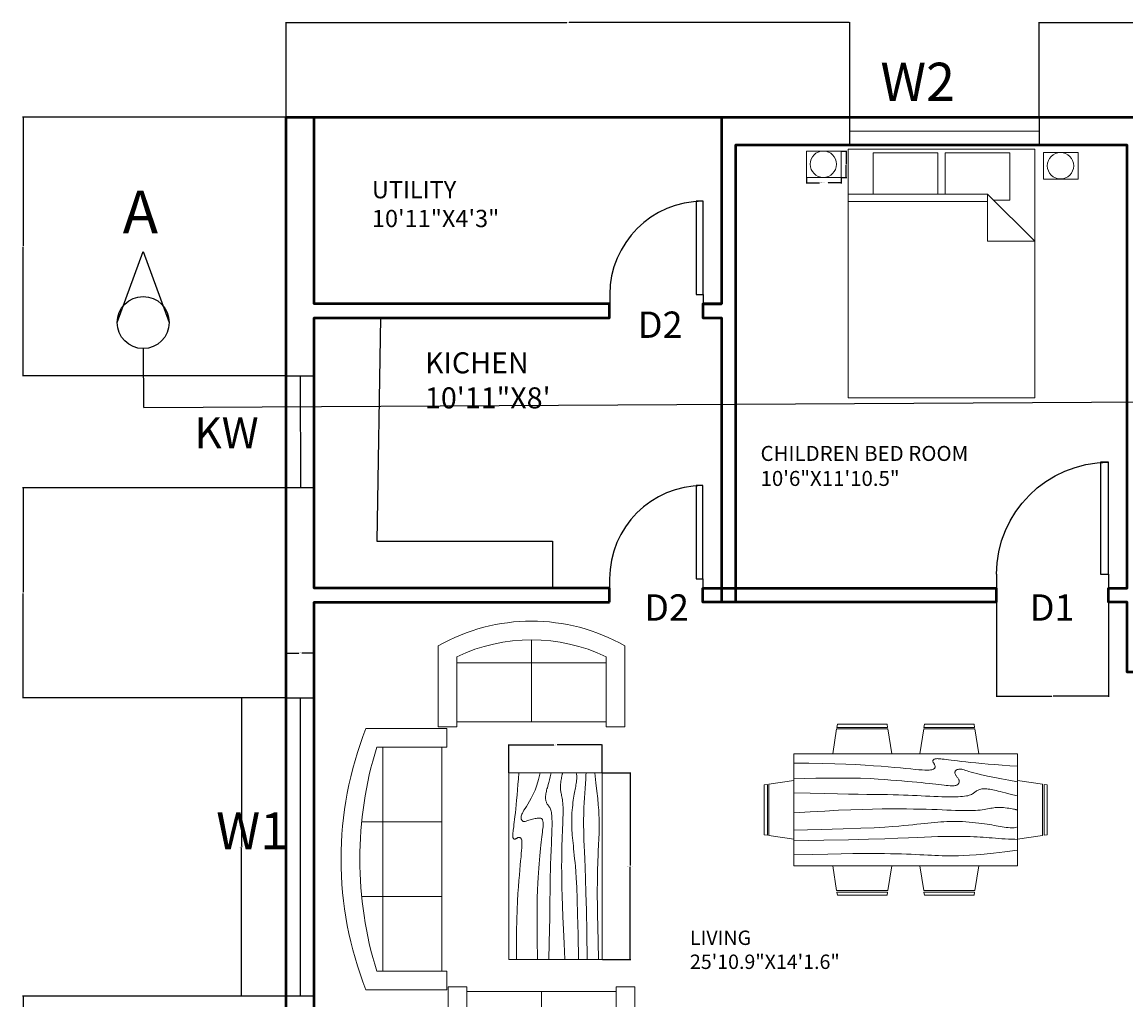
# Model space of a CAD drawing. Units: inches. Extents: x -45 to 1424, y 648 to 1662.
# Tile 2 of 8: x -45 to 310, y 896 to 1211. Entities that reach past the tile are written whole.
import ezdxf

# ---------------------------------------------------------------- set-up
doc = ezdxf.new("R2010")
doc.units = ezdxf.units.IN
for name, color, linetype, lineweight in [('A-ANNO-DIMS', 2, 'Continuous', 18), ('A-ANNO-SYMB', 7, 'Continuous', 25), ('A-ANNO-TEXT', 7, 'Continuous', 18), ('A-AREA-IDEN', 7, 'Continuous', 18), ('A-FLOR-CASE', 3, 'Continuous', 25), ('DOOR', 2, 'Continuous', 25), ('FURNITURE', 3, 'Continuous', 18), ('WALL', 4, 'Continuous', 50), ('WINDOW', 1, 'Continuous', 25)]:
    doc.layers.add(name, color=color, linetype=linetype, lineweight=lineweight)
doc.styles.get("Standard").update_dxf_attribs({"font": 'arial.ttf'})
doc.dimstyles.get("Standard").update_dxf_attribs({"dimtxt": 0.18, "dimasz": 0.18, "dimexe": 0.18, "dimexo": 0.0625, "dimgap": 0.09, "dimtad": 0, "dimtih": 1, "dimtoh": 1, "dimdec": 4, "dimzin": 0, "dimdsep": 46, "dimtxsty": 'Standard', "dimcen": 0.09, "dimadec": 0, "dimazin": 0, "dimtfac": 1, "dimtdec": 4, "dimtofl": 0, "dimtmove": 0, "dimatfit": 3, "dimfxl": 1, "dimtolj": 1, "dimtzin": 0, "dimarcsym": 0})

# ---------------------------------------------------------------- blocks, each defined once
blk = doc.blocks.new('*U2')
for p, q in [((-24, 0), (-24, -6)), ((0, 0), (0, -6))]:
    blk.add_line(p, q)
blk.add_lwpolyline([(0, 0), (0, 24), (-1.75, 24), (-1.75, 0)], close=True)
blk.add_arc((0, 0), 24, 90, 180)
blk = doc.blocks.new('*U3')
for p, q in [((0, 0), (0, -6)), ((24, 0), (24, -6))]:
    blk.add_line(p, q)
blk.add_lwpolyline([(0, 0), (0, 24), (1.75, 24), (1.75, 0)], close=True)
blk.add_arc((0, 0), 24, 0, 90)
blk = doc.blocks.new('Bed - Queen')
for p, q in [((0, -80.00003), (0, 0)), ((0, 0), (59.99999, 0)), ((59.99999, 0), (59.99999, -80.00003)), ((7.99999, -1.2), (28.79998, -1.2)), ((7.99999, -14.4), (7.99999, -1.2)), ((28.79998, -1.2), (28.79998, -14.4)), ((31.19999, -1.2), (51.99999, -1.2)), ((31.19999, -14.4), (31.19999, -1.2)), ((51.99999, -1.2), (51.99999, -16.4)), ((0, -14.4), (44.8, -14.4)), ((44.8, -16.8), (0, -16.8)), ((59.99999, -29.6), (44.8, -14.4)), ((44.8, -14.4), (44.8, -29.6)), ((51.99999, -16.4), (46.79936, -16.4)), ((44.8, -29.6), (59.99999, -29.6)), ((59.99999, -80.00003), (0, -80.00003))]:
    blk.add_line(p, q)
blk = doc.blocks.new('Sofa - Roundback 7 ft.')
for p, q in [((-12.00002, -32.4421), (-12.00003, -6.5971)), ((11.99997, -32.4421), (11.99998, -6.5971)), ((-36.000027, -34), (-36.000027, -11.4696)), ((-35.999844, -13.3819), (35.9998, -13.3819)), ((35.99998, -34), (35.99998, -11.4696)), ((-36.000027, -32.4421), (35.99998, -32.4421))]:
    blk.add_line(p, q)
for points in [[(-36.000027, -34), (-42.000027, -34), (-42.000027, -8)], [(41.99998, -8), (41.99998, -34), (35.99998, -34)]]:
    blk.add_lwpolyline(points)
for centre, radius, start, end in [((0, -114.25), 114.25, 68.43141, 111.5686), ((-0.00001, -127.1968), 121.1968, 72.72033, 107.2797)]:
    blk.add_arc(centre, radius, start, end)
blk = doc.blocks.new('Sofa - Roundback Loveseat 5 ft.')
for p, q in [((0, -32.44198), (0, -5.99998)), ((-24, -33.99998), (-24, -11.46958)), ((-23.9998, -13.38178), (23.99986, -13.38178)), ((24.00004, -33.99998), (24.00004, -11.46958)), ((-24, -32.44198), (24.00004, -32.44198))]:
    blk.add_line(p, q)
for points in [[(-24, -33.99998), (-30, -33.99998), (-30, -7.99998)], [(30.00004, -7.99998), (30.00004, -33.99998), (24.00004, -33.99998)]]:
    blk.add_lwpolyline(points)
for centre, radius, start, end in [((0, -60.24998), 60.24998, 60.13715, 119.8628), ((0, -61.38438), 55.38444, 64.32083, 115.6792)]:
    blk.add_arc(centre, radius, start, end)
blk = doc.blocks.new('Table - Rectangular Woodgrain 60 x 30 in.')
for p, q in [((0, 0), (0, -30)), ((60, 0), (0, 0)), ((60, -30), (60, 0)), ((0, -30), (60, -30))]:
    blk.add_line(p, q)
for points in [[(0, -2.4), (4.8155, -2.418), (9.0302, -2.4688), (12.709, -2.5477), (15.9167, -2.65), (18.7181, -2.7711), (21.1781, -2.9063), (23.3616, -3.0508), (25.3333, -3.2), (27.1477, -3.3495), (28.8172, -3.4958), (30.3437, -3.636), (31.7291, -3.7667), (32.9756, -3.8849), (34.0849, -3.9875), (35.059, -4.0714), (35.9, -4.1334), (36.6114, -4.1711), (37.2041, -4.1854), (37.6906, -4.1779), (38.0833, -4.15), (38.3948, -4.1034), (38.6375, -4.0396), (38.8239, -3.9602), (38.9666, -3.8667), (39.0764, -3.7608), (39.1573, -3.6448), (39.2116, -3.521), (39.2416, -3.3917), (39.2498, -3.2593), (39.2385, -3.1261), (39.21, -2.9944), (39.1666, -2.8667), (39.111, -2.7447), (39.0468, -2.6281), (38.978, -2.5163), (38.9083, -2.4083), (38.8418, -2.3035), (38.7823, -2.201), (38.7337, -2.1001), (38.7, -2), (38.6844, -1.9003), (38.6875, -1.8021), (38.7094, -1.707), (38.75, -1.6167), (38.8094, -1.5326), (38.8875, -1.4563), (38.9844, -1.3893), (39.1, -1.3333), (39.2351, -1.2896), (39.3937, -1.2583), (39.5804, -1.2396), (39.8, -1.2333), (40.057, -1.2396), (40.3562, -1.2583), (40.7023, -1.2896), (41.1, -1.3333), (41.5547, -1.3895), (42.0755, -1.4573), (42.6721, -1.5361), (43.3542, -1.625), (44.1316, -1.7233), (45.014, -1.8302), (46.0114, -1.9449), (47.1333, -2.0667), (48.3862, -2.1947), (49.7625, -2.3281), (51.2513, -2.4663), (52.8416, -2.6083), (54.5226, -2.7535), (56.2833, -2.9011), (58.1127, -3.0501), (60, -3.2)], [(0, -9.2), (6.5759, -9.0858), (11.9385, -9.0365), (16.2527, -9.0418), (19.6833, -9.0917), (22.3952, -9.1759), (24.5531, -9.2844), (26.322, -9.4069), (27.8666, -9.5333), (29.3241, -9.6553), (30.7203, -9.7719), (32.0532, -9.8837), (33.3208, -9.9917), (34.5213, -10.0965), (35.6526, -10.199), (36.7128, -10.2999), (37.7, -10.4), (38.6129, -10.4996), (39.4531, -10.5969), (40.223, -10.6895), (40.925, -10.775), (41.5613, -10.8512), (42.1344, -10.9156), (42.6465, -10.966), (43.1, -11), (43.4976, -11.0158), (43.8437, -11.0136), (44.143, -10.9942), (44.4, -10.9583), (44.6195, -10.9069), (44.8062, -10.8406), (44.9648, -10.7603), (45.1, -10.6667), (45.2155, -10.5598), (45.3114, -10.4365), (45.3871, -10.2929), (45.4416, -10.125), (45.4743, -9.929), (45.4844, -9.7011), (45.4709, -9.4371), (45.4333, -9.1333), (45.3716, -8.7883), (45.2896, -8.4104), (45.1919, -8.0107), (45.0833, -7.6), (44.9685, -7.1893), (44.8521, -6.7896), (44.7388, -6.4117), (44.6333, -6.0667), (44.54, -5.7628), (44.4614, -5.4979), (44.4001, -5.2675), (44.3583, -5.0667), (44.3384, -4.8909), (44.3427, -4.7354), (44.3736, -4.5956), (44.4333, -4.4667), (44.5236, -4.3453), (44.6427, -4.2333), (44.7884, -4.1339), (44.9583, -4.05), (45.1501, -3.9849), (45.3614, -3.9417), (45.59, -3.9234), (45.8333, -3.9333), (46.0915, -3.9749), (46.3734, -4.0531), (46.6906, -4.1736), (47.0542, -4.3417), (47.4756, -4.5629), (47.9661, -4.8427), (48.5372, -5.1866), (49.2, -5.6), (49.9676, -6.0844), (50.8594, -6.625), (51.8965, -7.2031), (53.1, -7.8), (54.491, -8.3969), (56.0906, -8.975), (57.9199, -9.5156), (60, -10)], [(0, -12.8), (5.1847, -12.9322), (9.6213, -13.0323), (13.3963, -13.1059), (16.5958, -13.1583), (19.3063, -13.1952), (21.614, -13.2219), (23.6054, -13.2439), (25.3666, -13.2667), (26.9728, -13.2947), (28.4531, -13.3281), (29.8256, -13.3663), (31.1083, -13.4083), (32.3191, -13.4535), (33.476, -13.501), (34.597, -13.5501), (35.7, -13.6), (36.7984, -13.6497), (37.8875, -13.6979), (38.9578, -13.743), (40, -13.7833), (41.0047, -13.8174), (41.9625, -13.8438), (42.864, -13.8607), (43.7, -13.8667), (44.4631, -13.8604), (45.1552, -13.8417), (45.7801, -13.8104), (46.3416, -13.7667), (46.8439, -13.7104), (47.2906, -13.6417), (47.6858, -13.5604), (48.0333, -13.4667), (48.3375, -13.3608), (48.6042, -13.2448), (48.8396, -13.121), (49.05, -12.9917), (49.2417, -12.8593), (49.4208, -12.7261), (49.5937, -12.5944), (49.7667, -12.4667), (49.9452, -12.3451), (50.1323, -12.2313), (50.3303, -12.1268), (50.5416, -12.0333), (50.7686, -11.9524), (51.0135, -11.8854), (51.2788, -11.8341), (51.5666, -11.8), (51.8785, -11.7843), (52.2116, -11.7865), (52.562, -11.8059), (52.926, -11.8417), (53.2998, -11.8931), (53.6795, -11.9594), (54.0614, -12.0397), (54.4416, -12.1333), (54.8223, -12.2401), (55.2293, -12.3625), (55.6942, -12.5037), (56.2489, -12.6667), (56.9251, -12.8547), (57.7545, -13.0708), (58.7689, -13.3182), (60, -13.6)], [(0, -18), (5.124, -17.7273), (9.6609, -17.5057), (13.6705, -17.3303), (17.2125, -17.1958), (20.3467, -17.0973), (23.1328, -17.0297), (25.6307, -16.9878), (27.9, -16.9667), (29.9928, -16.9617), (31.9302, -16.9703), (33.7254, -16.9907), (35.3917, -17.0208), (36.9423, -17.0588), (38.3906, -17.1026), (39.7499, -17.1503), (41.0333, -17.2), (42.2519, -17.2496), (43.4073, -17.2969), (44.4986, -17.3395), (45.525, -17.375), (46.4858, -17.4012), (47.3802, -17.4156), (48.2074, -17.416), (48.9667, -17.4), (49.6583, -17.3662), (50.2872, -17.3167), (50.8595, -17.2547), (51.3812, -17.1833), (51.8584, -17.1057), (52.2971, -17.025), (52.7034, -16.9443), (53.0833, -16.8667), (53.443, -16.7951), (53.789, -16.7313), (54.128, -16.6768), (54.4666, -16.6334), (54.8115, -16.6024), (55.1693, -16.5854), (55.5465, -16.5841), (55.95, -16.6), (56.3828, -16.6337), (56.8346, -16.6823), (57.2915, -16.7418), (57.7396, -16.8084), (58.165, -16.878), (58.5539, -16.9469), (58.8924, -17.0111), (59.1666, -17.0667), (59.3679, -17.1107), (59.5078, -17.1438), (59.6032, -17.1675), (59.6708, -17.1833), (59.7275, -17.193), (59.7901, -17.1979), (59.8753, -17.1998), (60, -17.2)], [(0, -22.4), (8.0098, -22.2501), (14.4094, -22.1011), (19.4168, -21.9535), (23.25, -21.8083), (26.1269, -21.6663), (28.2656, -21.5281), (29.884, -21.3947), (31.2, -21.2667), (32.3967, -21.1448), (33.5172, -21.0292), (34.5697, -20.9198), (35.5625, -20.8167), (36.5037, -20.7198), (37.4015, -20.6292), (38.2642, -20.5448), (39.1, -20.4667), (39.9164, -20.3951), (40.7187, -20.3313), (41.5117, -20.2768), (42.3, -20.2333), (43.0883, -20.2024), (43.8812, -20.1854), (44.6836, -20.1841), (45.5, -20.2), (46.3328, -20.234), (47.1747, -20.2844), (48.0163, -20.3488), (48.8479, -20.425), (49.66, -20.5106), (50.4429, -20.6031), (51.1872, -20.7004), (51.8833, -20.8), (52.5246, -20.8999), (53.1166, -20.9995), (53.6681, -21.0983), (54.1875, -21.1958), (54.6834, -21.2919), (55.1646, -21.3859), (55.6394, -21.4777), (56.1167, -21.5667), (56.6028, -21.6515), (57.0961, -21.7266), (57.5929, -21.7852), (58.0896, -21.8208), (58.5823, -21.8268), (59.0674, -21.7964), (59.5412, -21.723), (60, -21.6)], [(0, -25.2), (8.6355, -25.0504), (15.7026, -24.9031), (21.4049, -24.7606), (25.9458, -24.625), (29.529, -24.4988), (32.3578, -24.3844), (34.6359, -24.284), (36.5667, -24.2), (38.3213, -24.1341), (39.9417, -24.0854), (41.437, -24.0523), (42.8167, -24.0333), (44.0901, -24.0268), (45.2667, -24.0313), (46.3557, -24.0451), (47.3667, -24.0667), (48.309, -24.0947), (49.1928, -24.1287), (50.0284, -24.168), (50.826, -24.2125), (51.5959, -24.2617), (52.3483, -24.3151), (53.0935, -24.3725), (53.8417, -24.4334), (54.6009, -24.497), (55.3699, -24.561), (56.1454, -24.6226), (56.9239, -24.6792), (57.7021, -24.7279), (58.4764, -24.7662), (59.2435, -24.7911), (60, -24.8)], [(0, -28.8), (5.6867, -28.6681), (10.45, -28.5698), (14.407, -28.5012), (17.675, -28.4584), (20.3711, -28.4374), (22.6125, -28.4344), (24.5164, -28.4455), (26.2, -28.4667), (27.762, -28.4947), (29.2276, -28.5281), (30.6033, -28.5663), (31.8958, -28.6084), (33.1118, -28.6535), (34.2578, -28.7011), (35.3405, -28.7501), (36.3666, -28.8), (37.3443, -28.8497), (38.288, -28.8974), (39.2137, -28.9412), (40.1375, -28.9792), (41.0753, -29.0093), (42.0432, -29.0297), (43.0572, -29.0384), (44.1333, -29.0333), (45.2936, -29.0114), (46.5843, -28.9641), (48.0579, -28.8816), (49.7666, -28.7542), (51.7629, -28.5721), (54.0989, -28.3255), (56.8272, -28.0048), (60, -27.6)]]:
    blk.add_lwpolyline(points)
blk = doc.blocks.new('Dining Set - 36 x 72 in.')
for p, q in [((-22.2343, 26.00059), (-23.4847, 17.99762)), ((-22.2304, 26), (-5.7608, 26)), ((-22, 27.5), (-22.1562, 26.50042)), ((-5.8416, 26.5), (-22.1534, 26.5)), ((-22, 27.5), (-6, 27.5)), ((-5.8437, 26.49966), (-6, 27.5)), ((-4.5152, 17.99762), (-5.7655, 25.99926)), ((5.7657, 26.00059), (4.5153, 17.99762)), ((5.7696, 26), (22.2392, 26)), ((6, 27.5), (5.8438, 26.50042)), ((22.1584, 26.5), (5.8466, 26.5)), ((6, 27.5), (22, 27.5)), ((22.1563, 26.49966), (22, 27.5)), ((23.4848, 17.99762), (22.2345, 25.99926)), ((36, 18), (-36, 18)), ((-36, 18), (-36, -18)), ((36, -18), (36, 18)), ((-45.5, 8), (-44.5004, 8.15617)), ((-45.5, 8), (-45.5, -8)), ((-44.5, -8.15843), (-44.5, 8.15338)), ((-44.0006, 8.23428), (-35.9976, 9.48474)), ((-44, 8.23041), (-44, -8.23915)), ((44.0006, 8.23428), (35.9976, 9.48474)), ((44, 8.23041), (44, -8.23915)), ((44.5, -8.15843), (44.5, 8.15338)), ((45.5, 8), (44.5005, 8.15617)), ((45.5, 8), (45.5, -8)), ((-44.4997, -8.15631), (-45.5, -8)), ((-35.9976, -9.48476), (-43.9993, -8.2345)), ((35.9976, -9.48476), (43.9993, -8.2345)), ((44.4997, -8.15631), (45.5, -8)), ((-36, -18), (36, -18)), ((-22.2343, -26.0006), (-23.4847, -17.99762)), ((-4.5152, -17.99762), (-5.7655, -25.99928)), ((5.7657, -26.0006), (4.5153, -17.99762)), ((23.4848, -17.99762), (22.2345, -25.99928)), ((-22.2304, -26), (-5.7608, -26)), ((-22, -27.5), (-22.1562, -26.50044)), ((-5.8416, -26.5), (-22.1534, -26.5)), ((-22, -27.5), (-6, -27.5)), ((-5.8437, -26.49967), (-6, -27.5)), ((5.7696, -26), (22.2392, -26)), ((6, -27.5), (5.8438, -26.50044)), ((22.1584, -26.5), (5.8466, -26.5)), ((6, -27.5), (22, -27.5)), ((22.1563, -26.49967), (22, -27.5))]:
    blk.add_line(p, q)
for points in [[(-36, 15), (-31.1772, 14.97754), (-26.8079, 14.91406), (-22.8538, 14.81543), (-19.276, 14.6875), (-16.0362, 14.53613), (-13.0957, 14.36718), (-10.4159, 14.18652), (-7.9583, 14), (-5.6904, 13.81315), (-3.6035, 13.63021), (-1.6954, 13.45508), (0.0365, 13.29166), (1.5945, 13.14388), (2.9811, 13.01562), (4.1988, 12.9108), (5.25, 12.83333), (6.1393, 12.78613), (6.8802, 12.76823), (7.4883, 12.77767), (7.9792, 12.8125), (8.3685, 12.87077), (8.6719, 12.95052), (8.9049, 13.0498), (9.0833, 13.16666), (9.2205, 13.29899), (9.3216, 13.44401), (9.3895, 13.59879), (9.4271, 13.76041), (9.4373, 13.92594), (9.4232, 14.09245), (9.3875, 14.257), (9.3333, 14.41666), (9.2638, 14.56917), (9.1836, 14.71484), (9.0975, 14.85465), (9.0104, 14.98958), (8.9272, 15.1206), (8.8529, 15.2487), (8.7922, 15.37483), (8.75, 15.5), (8.7305, 15.62467), (8.7344, 15.74739), (8.7617, 15.86621), (8.8125, 15.97916), (8.8867, 16.08431), (8.9844, 16.17968), (9.1055, 16.26334), (9.25, 16.33333), (9.4189, 16.38802), (9.6172, 16.42708), (9.8506, 16.45052), (10.125, 16.45833), (10.4463, 16.45052), (10.8203, 16.42708), (11.2529, 16.38802), (11.75, 16.33333), (12.3184, 16.26318), (12.9694, 16.17838), (13.7151, 16.07991), (14.5677, 15.96875), (15.5395, 15.84586), (16.6426, 15.71224), (17.8893, 15.56884), (19.2917, 15.41666), (20.859, 15.25667), (22.5879, 15.08984), (24.4721, 14.91715), (26.5052, 14.73958), (28.6809, 14.5581), (30.9929, 14.3737), (33.4347, 14.18733), (36, 14)], [(-36, 10), (-28.9766, 10.14274), (-23.1725, 10.20442), (-18.4241, 10.19775), (-14.5677, 10.13541), (-11.4399, 10.03011), (-8.877, 9.89453), (-6.7154, 9.74137), (-4.7917, 9.58333), (-2.9698, 9.43082), (-1.2246, 9.28515), (0.4415, 9.14534), (2.026, 9.01041), (3.5266, 8.87939), (4.9408, 8.7513), (6.266, 8.62516), (7.5, 8.5), (8.6411, 8.37549), (9.6914, 8.2539), (10.6538, 8.13818), (11.5312, 8.03125), (12.3267, 7.93603), (13.043, 7.85547), (13.6831, 7.79248), (14.25, 7.75), (14.7471, 7.7303), (15.1797, 7.73307), (15.5537, 7.75732), (15.875, 7.80208), (16.1494, 7.86637), (16.3828, 7.94922), (16.5811, 8.04964), (16.75, 8.16666), (16.8944, 8.29915), (17.0143, 8.44531), (17.1089, 8.60319), (17.1771, 8.77083), (17.218, 8.94629), (17.2305, 9.1276), (17.2137, 9.31282), (17.1667, 9.5), (17.0895, 9.6875), (16.987, 9.875), (16.8649, 10.0625), (16.7292, 10.25), (16.5856, 10.4375), (16.4401, 10.625), (16.2985, 10.8125), (16.1667, 11), (16.05, 11.18733), (15.9518, 11.3737), (15.8752, 11.5581), (15.8229, 11.73958), (15.798, 11.91715), (15.8034, 12.08984), (15.842, 12.25667), (15.9167, 12.41666), (16.0295, 12.56836), (16.1784, 12.70833), (16.3605, 12.83268), (16.5729, 12.9375), (16.8127, 13.01888), (17.0768, 13.07291), (17.3625, 13.0957), (17.6667, 13.08333), (17.9894, 13.03312), (18.3418, 12.94726), (18.7382, 12.82918), (19.1927, 12.68229), (19.7195, 12.51001), (20.3327, 12.31575), (21.0465, 12.10294), (21.875, 11.875), (22.8357, 11.63354), (23.959, 11.37304), (25.2786, 11.08618), (26.8282, 10.76562), (28.6414, 10.40405), (30.752, 9.99414), (33.1936, 9.52856), (36, 9)], [(-36, 5.5), (-30.7157, 5.3348), (-26.069, 5.20963), (-21.9946, 5.11767), (-18.4271, 5.05208), (-15.3009, 5.00602), (-12.5508, 4.97265), (-10.1112, 4.94515), (-7.9167, 4.91666), (-5.909, 4.88167), (-4.0586, 4.83984), (-2.3429, 4.79215), (-0.7396, 4.73958), (0.7739, 4.6831), (2.22, 4.6237), (3.6213, 4.56233), (5, 4.5), (6.373, 4.43782), (7.7344, 4.3776), (9.0723, 4.32129), (10.375, 4.27083), (11.6309, 4.22819), (12.8281, 4.19531), (13.9551, 4.17415), (15, 4.16666), (15.954, 4.17448), (16.819, 4.19791), (17.6001, 4.23698), (18.3021, 4.29166), (18.9299, 4.36198), (19.4883, 4.44791), (19.9823, 4.54948), (20.4167, 4.66666), (20.7969, 4.79899), (21.1302, 4.94401), (21.4245, 5.09879), (21.6875, 5.26041), (21.9271, 5.42594), (22.1511, 5.59245), (22.3672, 5.757), (22.5834, 5.91666), (22.8065, 6.06868), (23.0404, 6.21093), (23.2879, 6.34147), (23.5521, 6.45833), (23.8358, 6.55957), (24.142, 6.64323), (24.4735, 6.70735), (24.8334, 6.75), (25.2235, 6.76969), (25.642, 6.76692), (26.0858, 6.74267), (26.5521, 6.69791), (27.0379, 6.63362), (27.5404, 6.55078), (28.0565, 6.45036), (28.5834, 6.33333), (29.1242, 6.19987), (29.7071, 6.04687), (30.3661, 5.87044), (31.1354, 5.66666), (32.0493, 5.43164), (33.142, 5.16146), (34.4475, 4.85221), (36, 4.5)], [(-36, -1), (-30.7915, -0.6591), (-26.0195, -0.38216), (-21.6519, -0.16284), (-17.6563, 0.00521), (-14.0005, 0.12833), (-10.6523, 0.21289), (-7.5796, 0.26522), (-4.75, 0.29166), (-2.134, 0.29793), (0.2878, 0.28711), (2.5317, 0.26163), (4.6146, 0.22396), (6.5529, 0.17651), (8.3633, 0.12174), (10.0623, 0.06209), (11.6667, 0), (13.1899, -0.06201), (14.6341, -0.1211), (15.9982, -0.17432), (17.2813, -0.21875), (18.4823, -0.25147), (19.6003, -0.26953), (20.6343, -0.27002), (21.5834, -0.25), (22.4481, -0.20768), (23.2357, -0.14584), (23.9549, -0.06836), (24.6146, 0.02083), (25.2235, 0.11784), (25.7904, 0.21875), (26.3241, 0.31966), (26.8334, 0.41666), (27.3265, 0.50618), (27.8099, 0.58593), (28.2894, 0.65397), (28.7709, 0.70833), (29.2601, 0.74707), (29.763, 0.76823), (30.2855, 0.76985), (30.8334, 0.75), (31.4088, 0.70784), (31.9994, 0.64713), (32.589, 0.57275), (33.1615, 0.48958), (33.7008, 0.4025), (34.1908, 0.3164), (34.6153, 0.23616), (34.9584, 0.16666), (35.2099, 0.11165), (35.3848, 0.07031), (35.504, 0.04069), (35.5886, 0.02083), (35.6594, 0.00879), (35.7377, 0.0026), (35.8442, 0.00032), (36, 0)], [(-36, -6.5), (-27.1843, -6.31267), (-20.084, -6.1263), (-14.469, -5.9419), (-10.1094, -5.76042), (-6.7752, -5.58285), (-4.2363, -5.41016), (-2.2629, -5.24333), (-0.625, -5.08334), (0.8708, -4.93099), (2.2715, -4.78646), (3.5872, -4.64974), (4.8281, -4.52084), (6.0046, -4.39974), (7.127, -4.28646), (8.2053, -4.18099), (9.25, -4.08334), (10.2705, -3.99382), (11.2734, -3.91407), (12.2647, -3.84603), (13.25, -3.79167), (14.2354, -3.75293), (15.2266, -3.73177), (16.2295, -3.73015), (17.25, -3.75), (18.2912, -3.79248), (19.3451, -3.85547), (20.4009, -3.93604), (21.4479, -4.03125), (22.4754, -4.13819), (23.4727, -4.25391), (24.4289, -4.37549), (25.3334, -4.5), (26.1785, -4.62492), (26.9694, -4.74935), (27.7145, -4.87281), (28.4219, -4.99479), (29.1, -5.11483), (29.7572, -5.23242), (30.4016, -5.34709), (31.0417, -5.45834), (31.6837, -5.56437), (32.3262, -5.65821), (32.9658, -5.73153), (33.599, -5.77604), (34.2224, -5.78345), (34.8327, -5.74545), (35.4264, -5.65373), (36, -5.5)], [(-36, -10), (-26.4022, -9.81299), (-18.4675, -9.62891), (-11.9839, -9.45069), (-6.7396, -9.28125), (-2.5226, -9.12354), (0.8789, -8.98047), (3.6769, -8.85498), (6.0833, -8.75), (8.2767, -8.66765), (10.3021, -8.60677), (12.1712, -8.56543), (13.8958, -8.54167), (15.4876, -8.53353), (16.9583, -8.53907), (18.3197, -8.55632), (19.5834, -8.58334), (20.7616, -8.61841), (21.8685, -8.66081), (22.9188, -8.71004), (23.9271, -8.76563), (24.9081, -8.82707), (25.8763, -8.89388), (26.8465, -8.96558), (27.8334, -9.04167), (28.8474, -9.12118), (29.8828, -9.20117), (30.93, -9.27824), (31.9792, -9.34896), (33.0205, -9.40991), (34.0443, -9.45768), (35.0407, -9.48885), (36, -9.5)], [(-36, -14.5), (-30.0881, -14.33513), (-25.0332, -14.21224), (-20.7312, -14.12647), (-17.0781, -14.07292), (-13.97, -14.04671), (-11.3027, -14.04297), (-8.9724, -14.05681), (-6.875, -14.08334), (-4.9224, -14.11833), (-3.0905, -14.16016), (-1.3709, -14.20785), (0.2448, -14.26042), (1.7647, -14.3169), (3.1973, -14.3763), (4.5507, -14.43767), (5.8333, -14.5), (7.0554, -14.5621), (8.235, -14.62175), (9.3922, -14.67652), (10.5469, -14.72396), (11.7192, -14.76164), (12.929, -14.78711), (14.1965, -14.79794), (15.5417, -14.79167), (16.9933, -14.76424), (18.6152, -14.70508), (20.4804, -14.60197), (22.6615, -14.44271), (25.2312, -14.21509), (28.2624, -13.9069), (31.8277, -13.50594), (36, -13)]]:
    blk.add_lwpolyline(points)
blk = doc.blocks.new('WIN-W2-BEDROOM-N')
for p, q in [((0, 0), (0, 9)), ((0, 9), (60.88, 9)), ((60.88, 9.18), (60.88, 0)), ((0, 4.5), (60.88, 4.59)), ((60.88, 0), (0, 0))]:
    blk.add_line(p, q)
blk = doc.blocks.new('WIN-KW-KITCHEN')
for p, q in [((0, 36), (9, 36)), ((0, 0), (0, 36)), ((4.5, 36), (4.53, 0)), ((9, 36), (9.05, 0)), ((9.05, 0), (0, 0))]:
    blk.add_line(p, q)
blk = doc.blocks.new('WIN-W1-LIVING')
for p, q in [((0, 96), (9, 96)), ((0, 0), (0, 96)), ((4.5, 96), (4.5, 0)), ((8.72, 0), (9, 96)), ((8.72, 0), (0, 0))]:
    blk.add_line(p, q)
blk = doc.blocks.new('FURN-BEDSIDE-UNIT')
blk.add_lwpolyline([(0, 8.55), (11.15, 8.55), (11.15, 0), (0, 0)], close=True)
blk.add_circle((5.42, 4.31), 4.24)
blk = doc.blocks.new('CASEWORK-KITCHEN')
for p, q in [((1.26, 87), (0, 15.15)), ((0, 15.15), (56.6, 15.15)), ((56.6, 15.15), (56.6, 0))]:
    blk.add_line(p, q)
blk = doc.blocks.new('SECTION-DIRECTION')
for p, q in [((0, 27.32), (8.32, 50.22)), ((8.32, 50.22), (16.73, 27.32)), ((8.52, 0), (8.41, 18.95))]:
    blk.add_line(p, q)
blk.add_circle((8.36, 27.32), 8.36)
blk = doc.blocks.new('*D36')
at = {"layer": 'A-ANNO-DIMS', "color": 0, "lineweight": -2, "transparency": 16777216}
for p, q in [((207.34, 1160.5), (207.34, 1158.72)), ((207.52, 1158.9), (211.54, 1158.9)), ((218.31, 1158.9), (214.29, 1158.9)), ((218.49, 1160.5), (218.49, 1158.72))]:
    blk.add_line(p, q, dxfattribs=at)
at = {"layer": 'A-ANNO-DIMS', "color": 0, "transparency": 16777216}
for points in [[(207.52, 1158.93), (207.52, 1158.87), (207.34, 1158.9)], [(218.31, 1158.93), (218.31, 1158.87), (218.49, 1158.9)]]:
    blk.add_solid(points, dxfattribs=at)
at = {"layer": 'Defpoints', "color": 0, "transparency": 16777216}
for p in [(207.34, 1160.57), (218.49, 1160.57), (218.49, 1158.9)]:
    blk.add_point(p, dxfattribs=at)
at = {"layer": 'A-ANNO-DIMS', "color": 0, "transparency": 16777216, "insert": (212.92, 1158.9), "char_height": 0.18, "attachment_point": 5}
blk.add_mtext('\\A1;NIGHTSTAND 11 TYP.', dxfattribs=at)
blk = doc.blocks.new('*D37')
at = {"layer": 'A-ANNO-DIMS', "color": 0, "lineweight": -2, "transparency": 16777216}
for p, q in [((218.55, 1169.12), (220.34, 1169.12)), ((220.16, 1168.94), (220.16, 1165.02)), ((220.16, 1160.75), (220.16, 1164.66)), ((218.55, 1160.57), (220.34, 1160.57))]:
    blk.add_line(p, q, dxfattribs=at)
at = {"layer": 'A-ANNO-DIMS', "color": 0, "transparency": 16777216}
for points in [[(220.13, 1168.94), (220.19, 1168.94), (220.16, 1169.12)], [(220.13, 1160.75), (220.19, 1160.75), (220.16, 1160.57)]]:
    blk.add_solid(points, dxfattribs=at)
at = {"layer": 'Defpoints', "color": 0, "transparency": 16777216}
for p in [(218.49, 1169.12), (220.16, 1169.12), (218.49, 1160.57)]:
    blk.add_point(p, dxfattribs=at)
at = {"layer": 'A-ANNO-DIMS', "color": 0, "transparency": 16777216, "insert": (220.16, 1164.84), "char_height": 0.18, "attachment_point": 5}
blk.add_mtext('\\A1;9 TYP.', dxfattribs=at)
blk = doc.blocks.new('*D44')
at = {"layer": 'A-ANNO-DIMS', "color": 0, "lineweight": -2, "transparency": 16777216}
for p, q in [((141.68, 969.1), (150.8, 969.1)), ((150.62, 968.92), (150.62, 939.28)), ((150.62, 909.28), (150.62, 938.92)), ((141.68, 909.1), (150.8, 909.1))]:
    blk.add_line(p, q, dxfattribs=at)
at = {"layer": 'A-ANNO-DIMS', "color": 0, "transparency": 16777216}
for points in [[(150.59, 968.92), (150.65, 968.92), (150.62, 969.1)], [(150.59, 909.28), (150.65, 909.28), (150.62, 909.1)]]:
    blk.add_solid(points, dxfattribs=at)
at = {"layer": 'Defpoints', "color": 0, "transparency": 16777216}
for p in [(141.62, 969.1), (150.62, 969.1), (141.62, 909.1)]:
    blk.add_point(p, dxfattribs=at)
at = {"layer": 'A-ANNO-DIMS', "color": 0, "transparency": 16777216, "insert": (150.62, 939.1), "char_height": 0.18, "attachment_point": 5}
blk.add_mtext('\\A1;COFFEE TABLE 60 TYP.', dxfattribs=at)
blk = doc.blocks.new('*D45')
at = {"layer": 'A-ANNO-DIMS', "color": 0, "lineweight": -2, "transparency": 16777216}
for p, q in [((111.62, 969.16), (111.62, 978.28)), ((111.8, 978.1), (126.09, 978.1)), ((141.44, 978.1), (127.15, 978.1)), ((141.62, 969.16), (141.62, 978.28))]:
    blk.add_line(p, q, dxfattribs=at)
at = {"layer": 'A-ANNO-DIMS', "color": 0, "transparency": 16777216}
for points in [[(111.8, 978.13), (111.8, 978.07), (111.62, 978.1)], [(141.44, 978.13), (141.44, 978.07), (141.62, 978.1)]]:
    blk.add_solid(points, dxfattribs=at)
at = {"layer": 'Defpoints', "color": 0, "transparency": 16777216}
for p in [(111.62, 978.1), (111.62, 969.1), (141.62, 969.1)]:
    blk.add_point(p, dxfattribs=at)
at = {"layer": 'A-ANNO-DIMS', "color": 0, "transparency": 16777216, "insert": (126.62, 978.1), "char_height": 0.18, "attachment_point": 5}
blk.add_mtext('\\A1;30 TYP.', dxfattribs=at)
blk = doc.blocks.new('*D60')
at = {"layer": 'A-ANNO-DIMS', "color": 0, "lineweight": -2, "transparency": 16777216}
for p, q in [((39.94, 993.23), (25.42, 993.23)), ((25.6, 993.05), (25.6, 945.42)), ((25.6, 897.41), (25.6, 945.05)), ((39.94, 897.23), (25.42, 897.23))]:
    blk.add_line(p, q, dxfattribs=at)
at = {"layer": 'A-ANNO-DIMS', "color": 0, "transparency": 16777216}
for points in [[(25.57, 993.05), (25.63, 993.05), (25.6, 993.23)], [(25.57, 897.41), (25.63, 897.41), (25.6, 897.23)]]:
    blk.add_solid(points, dxfattribs=at)
at = {"layer": 'Defpoints', "color": 0, "transparency": 16777216}
for p in [(25.6, 993.23), (40, 993.23), (40, 897.23)]:
    blk.add_point(p, dxfattribs=at)
at = {"layer": 'A-ANNO-DIMS', "color": 0, "transparency": 16777216, "insert": (25.6, 945.23), "char_height": 0.18, "attachment_point": 5}
blk.add_mtext('\\A1;W1 96 TYP.', dxfattribs=at)
blk = doc.blocks.new('*D61')
at = {"layer": 'A-ANNO-DIMS', "color": 0, "lineweight": -2, "transparency": 16777216}
for p, q in [((40, 993.3), (40, 1007.81)), ((40.18, 1007.63), (44.04, 1007.63)), ((48.82, 1007.63), (44.96, 1007.63)), ((49, 993.3), (49, 1007.81))]:
    blk.add_line(p, q, dxfattribs=at)
at = {"layer": 'A-ANNO-DIMS', "color": 0, "transparency": 16777216}
for points in [[(40.18, 1007.66), (40.18, 1007.6), (40, 1007.63)], [(48.82, 1007.66), (48.82, 1007.6), (49, 1007.63)]]:
    blk.add_solid(points, dxfattribs=at)
at = {"layer": 'Defpoints', "color": 0, "transparency": 16777216}
for p in [(49, 1007.63), (40, 993.23), (49, 993.23)]:
    blk.add_point(p, dxfattribs=at)
at = {"layer": 'A-ANNO-DIMS', "color": 0, "transparency": 16777216, "insert": (44.5, 1007.63), "char_height": 0.18, "attachment_point": 5}
blk.add_mtext('\\A1;9 TYP.', dxfattribs=at)
blk = doc.blocks.new('*D76')
at = {"layer": 'A-ANNO-DIMS', "color": 0, "lineweight": -2, "transparency": 16777216}
for p, q in [((40, 1180.06), (40, 1210.61)), ((40.18, 1210.43), (130.26, 1210.43)), ((221.1, 1210.43), (131.03, 1210.43)), ((221.28, 1180.06), (221.28, 1210.61))]:
    blk.add_line(p, q, dxfattribs=at)
at = {"layer": 'A-ANNO-DIMS', "color": 0, "transparency": 16777216}
for points in [[(40.18, 1210.46), (40.18, 1210.4), (40, 1210.43)], [(221.1, 1210.46), (221.1, 1210.4), (221.28, 1210.43)]]:
    blk.add_solid(points, dxfattribs=at)
at = {"layer": 'Defpoints', "color": 0, "transparency": 16777216}
for p in [(221.28, 1210.43), (40, 1180), (221.28, 1180)]:
    blk.add_point(p, dxfattribs=at)
at = {"layer": 'A-ANNO-DIMS', "color": 0, "transparency": 16777216, "insert": (130.64, 1210.43), "char_height": 0.18, "attachment_point": 5}
blk.add_mtext('\\A1;181.3', dxfattribs=at)
blk = doc.blocks.new('*D77')
at = {"layer": 'A-ANNO-DIMS', "color": 0, "lineweight": -2, "transparency": 16777216}
for p, q in [((282.16, 1180.06), (282.16, 1210.61)), ((282.34, 1210.43), (316.83, 1210.43)), ((352.1, 1210.43), (317.61, 1210.43)), ((352.28, 1180.06), (352.28, 1210.61))]:
    blk.add_line(p, q, dxfattribs=at)
at = {"layer": 'A-ANNO-DIMS', "color": 0, "transparency": 16777216}
for points in [[(282.34, 1210.46), (282.34, 1210.4), (282.16, 1210.43)], [(352.1, 1210.46), (352.1, 1210.4), (352.28, 1210.43)]]:
    blk.add_solid(points, dxfattribs=at)
at = {"layer": 'Defpoints', "color": 0, "transparency": 16777216}
for p in [(352.28, 1210.43), (282.16, 1180), (352.28, 1180)]:
    blk.add_point(p, dxfattribs=at)
at = {"layer": 'A-ANNO-DIMS', "color": 0, "transparency": 16777216, "insert": (317.22, 1210.43), "char_height": 0.18, "attachment_point": 5}
blk.add_mtext('\\A1;70.12', dxfattribs=at)
blk = doc.blocks.new('*D81')
at = {"layer": 'A-ANNO-DIMS', "color": 0, "lineweight": -2, "transparency": 16777216}
for p, q in [((268.5, 1023.94), (268.5, 993.57)), ((304.5, 1023.94), (304.5, 993.57)), ((268.68, 993.75), (286.28, 993.75)), ((304.32, 993.75), (286.72, 993.75))]:
    blk.add_line(p, q, dxfattribs=at)
at = {"layer": 'A-ANNO-DIMS', "color": 0, "transparency": 16777216}
for points in [[(268.68, 993.78), (268.68, 993.72), (268.5, 993.75)], [(304.32, 993.78), (304.32, 993.72), (304.5, 993.75)]]:
    blk.add_solid(points, dxfattribs=at)
at = {"layer": 'Defpoints', "color": 0, "transparency": 16777216}
for p in [(268.5, 1024), (304.5, 1024), (268.5, 993.75)]:
    blk.add_point(p, dxfattribs=at)
at = {"layer": 'A-ANNO-DIMS', "color": 0, "transparency": 16777216, "insert": (286.5, 993.75), "char_height": 0.18, "attachment_point": 5}
blk.add_mtext('\\A1;36', dxfattribs=at)
blk = doc.blocks.new('*D88')
at = {"layer": 'A-ANNO-DIMS', "color": 0, "lineweight": -2, "transparency": 16777216}
for p, q in [((39.94, 897.23), (-44.82, 897.23)), ((-44.64, 897.05), (-44.64, 862.46)), ((-44.64, 827.51), (-44.64, 862.1)), ((39.94, 827.33), (-44.82, 827.33))]:
    blk.add_line(p, q, dxfattribs=at)
at = {"layer": 'A-ANNO-DIMS', "color": 0, "transparency": 16777216}
for points in [[(-44.67, 897.05), (-44.61, 897.05), (-44.64, 897.23)], [(-44.67, 827.51), (-44.61, 827.51), (-44.64, 827.33)]]:
    blk.add_solid(points, dxfattribs=at)
at = {"layer": 'Defpoints', "color": 0, "transparency": 16777216}
for p in [(-44.64, 897.23), (40, 897.23), (40, 827.33)]:
    blk.add_point(p, dxfattribs=at)
at = {"layer": 'A-ANNO-DIMS', "color": 0, "transparency": 16777216, "insert": (-44.64, 862.28), "char_height": 0.18, "attachment_point": 5}
blk.add_mtext('\\A1;69.9', dxfattribs=at)
blk = doc.blocks.new('*D89')
at = {"layer": 'A-ANNO-DIMS', "color": 0, "lineweight": -2, "transparency": 16777216}
for p, q in [((39.94, 1060.79), (-44.82, 1060.79)), ((-44.64, 1060.61), (-44.64, 1027.19)), ((-44.64, 993.41), (-44.64, 1026.83)), ((39.94, 993.23), (-44.82, 993.23))]:
    blk.add_line(p, q, dxfattribs=at)
at = {"layer": 'A-ANNO-DIMS', "color": 0, "transparency": 16777216}
for points in [[(-44.67, 1060.61), (-44.61, 1060.61), (-44.64, 1060.79)], [(-44.67, 993.41), (-44.61, 993.41), (-44.64, 993.23)]]:
    blk.add_solid(points, dxfattribs=at)
at = {"layer": 'Defpoints', "color": 0, "transparency": 16777216}
for p in [(-44.64, 1060.79), (40, 1060.79), (40, 993.23)]:
    blk.add_point(p, dxfattribs=at)
at = {"layer": 'A-ANNO-DIMS', "color": 0, "transparency": 16777216, "insert": (-44.64, 1027.01), "char_height": 0.18, "attachment_point": 5}
blk.add_mtext('\\A1;67.56', dxfattribs=at)
blk = doc.blocks.new('*D90')
at = {"layer": 'A-ANNO-DIMS', "color": 0, "lineweight": -2, "transparency": 16777216}
for p, q in [((39.94, 1180), (-44.82, 1180)), ((-44.64, 1179.82), (-44.64, 1138.58)), ((-44.64, 1096.97), (-44.64, 1138.21)), ((39.94, 1096.79), (-44.82, 1096.79))]:
    blk.add_line(p, q, dxfattribs=at)
at = {"layer": 'A-ANNO-DIMS', "color": 0, "transparency": 16777216}
for points in [[(-44.67, 1179.82), (-44.61, 1179.82), (-44.64, 1180)], [(-44.67, 1096.97), (-44.61, 1096.97), (-44.64, 1096.79)]]:
    blk.add_solid(points, dxfattribs=at)
at = {"layer": 'Defpoints', "color": 0, "transparency": 16777216}
for p in [(-44.64, 1180), (40, 1180), (40, 1096.79)]:
    blk.add_point(p, dxfattribs=at)
at = {"layer": 'A-ANNO-DIMS', "color": 0, "transparency": 16777216, "insert": (-44.64, 1138.39), "char_height": 0.18, "attachment_point": 5}
blk.add_mtext('\\A1;83.21', dxfattribs=at)

msp = doc.modelspace()

# ---------------------------------------------------------------- linework, layer by layer
at = {"layer": 'A-ANNO-SYMB'}
msp.add_line((-5.8705, 1086.6362), (528.1294, 1089.7026), dxfattribs=at)
at = {"layer": 'WALL'}
for p, q in [((174, 1120), (180, 1120)), ((144.0001, 1024), (144.0001, 1028.5)), ((268.5002, 1024), (268.5002, 1028.5))]:
    msp.add_line(p, q, dxfattribs=at)
msp.add_lwpolyline([(465.4, 1180), (465.4, 712), (40, 712), (40, 1180)], close=True, dxfattribs=at)
for points in [[(144.0001, 1028.5), (49, 1028.5), (49, 1115.5), (144.0021, 1115.5), (144.0021, 1120), (49, 1120), (49, 1180)], [(180, 1180), (180, 1120), (174, 1120.0161), (174, 1115.5), (180, 1115.5), (180, 1024)], [(320.997, 1001.5), (310.5, 1001.5), (310.5, 1024), (304.5002, 1024), (304.5002, 1028.5), (310.5, 1028.5), (310.5, 1171), (184.5, 1171), (184.5, 1024)], [(268.5002, 1024), (174.0001, 1024), (174.0001, 1028.4666), (180, 1028.5), (268.5002, 1028.5)], [(279.9, 712), (279.9, 721), (279.7284, 774.2923), (270.9, 774.2923), (270.9, 721), (49, 721), (49, 849.9), (228.9004, 849.9), (228.9004, 854.4), (49, 854.4), (49, 1024), (144.0001, 1024)]]:
    msp.add_lwpolyline(points, dxfattribs=at)

# ---------------------------------------------------------------- block references
at = {"layer": 'A-ANNO-SYMB'}
msp.add_blockref('SECTION-DIRECTION', (-14.3908, 1086.6366), dxfattribs=at)
at = {"layer": 'A-FLOR-CASE'}
msp.add_blockref('CASEWORK-KITCHEN', (69.09, 1028.5), dxfattribs=at)
at = {"layer": 'DOOR'}
for name, p, xscale, yscale, zscale in [('*U2', (174.057, 1122.9841), 1.25, 1.25, 1.25), ('*U3', (304.5002, 1033), -1.5, 1.5, 1.5), ('*U2', (174.0001, 1031.5), 1.25, 1.25, 1.25)]:
    msp.add_blockref(name, p, dxfattribs=dict(at, xscale=xscale, yscale=yscale, zscale=zscale))
at = {"layer": 'FURNITURE'}
for name, p in [('FURN-BEDSIDE-UNIT', (207.342, 1160.567)), ('Bed - Queen', (220.7596, 1169.7061)), ('FURN-BEDSIDE-UNIT', (283.6387, 1160.0794)), ('Sofa - Roundback Loveseat 5 ft.', (118.905, 1017.917)), ('Dining Set - 36 x 72 in.', (239.277, 957.2156))]:
    msp.add_blockref(name, p, dxfattribs=at)
for name, p, rotation in [('Sofa - Roundback 7 ft.', (57.6335, 941.3265), 89.99999549093542), ('Table - Rectangular Woodgrain 60 x 30 in.', (111.6215, 909.0997), 89.99999999999976), ('Sofa - Roundback Loveseat 5 ft.', (122.0801, 866.3268), 180)]:
    msp.add_blockref(name, p, dxfattribs=dict(at, rotation=rotation))
at = {"layer": 'WINDOW'}
for name, p in [('WIN-W2-BEDROOM-N', (221.284, 1171)), ('WIN-KW-KITCHEN', (40, 1060.79)), ('WIN-W1-LIVING', (40, 897.234))]:
    msp.add_blockref(name, p, dxfattribs=at)

# ---------------------------------------------------------------- texts
at = {"layer": 'A-ANNO-SYMB', "insert": (-12.6337, 1156.3961), "char_height": 13.7453, "attachment_point": 1}
msp.add_mtext_dynamic_manual_height_columns('A', width=15.088715, gutter_width=68.7265, heights=[13.7453], dxfattribs=at)
at = {"layer": 'A-ANNO-TEXT', "insert": (231.1307, 1197.5355), "char_height": 12.26218, "width": 1.05025, "attachment_point": 1}
msp.add_mtext('W2', dxfattribs=at)
at = {"layer": 'A-ANNO-TEXT', "attachment_point": 1}
for s, width, gutter_width, heights, insert, char_height in [('D2', 4.069942, 42.3777, [0], (153.0977, 1117.4957), 8.47554), ('KW', 23.512637, 49.6518, [9.9304], (10.4669, 1083.4667), 9.93036), ('D2', 4.069942, 42.3777, [0], (155.1481, 1026.5304), 8.47554), ('D1', 8.475535, 42.3777, [0], (279.1882, 1026.5304), 8.47554), ('W1', 18.68524, 59.1031, [0], (17.4497, 956.3661), 11.82062)]:
    msp.add_mtext_dynamic_manual_height_columns(s, width=width, gutter_width=gutter_width, heights=heights, dxfattribs=dict(at, insert=insert, char_height=char_height))
at = {"layer": 'A-AREA-IDEN', "attachment_point": 1}
for s, width, gutter_width, insert, char_height in [('UTILITY\\P10\'11"X4\'3"', 7.386172, 26.803, (67.5327, 1159.4703), 5.556295), ('LIVING\\P25\'10.9"X14\'1.6"', 4.630949, 23.1547, (169.8433, 918.3767), 4.630949)]:
    msp.add_mtext_dynamic_manual_height_columns(s, width=width, gutter_width=gutter_width, heights=[0], dxfattribs=dict(at, insert=insert, char_height=char_height))
for s, insert, char_height in [('KICHEN\\P10\'11"X8\'', (84.612, 1104.3786), 6.76397), ('CHILDREN BED ROOM\\P10\'6"X11\'10.5"', (192.5652, 1074.2668), 4.825426)]:
    msp.add_mtext(s, dxfattribs=dict(at, insert=insert, char_height=char_height))

# ---------------------------------------------------------------- dimensions: what is measured, and where the dimension line sits
at = {"layer": 'A-ANNO-DIMS'}
for base, p1, p2, override, picture, middle in [((221.2841, 1210.4279), (40, 1180), (221.2841, 1180), {"dimdec": 1, "dimlfac": 1, "dimrnd": 0, "dimzin": 0, "dimdsep": 46, "dimlunit": 2}, '*D76', (130.6421, 1210.4279)), ((352.2766, 1210.4279), (282.1613, 1180), (352.2766, 1180), {"dimdec": 2, "dimlfac": 1, "dimrnd": 0, "dimzin": 0, "dimdsep": 46, "dimlunit": 2}, '*D77', (317.2189, 1210.4279))]:
    dim = msp.add_linear_dim(base=base, p1=p1, p2=p2, dimstyle='Standard', override=override, dxfattribs=at)
    dim.commit()
    dim.dimension.update_dxf_attribs({"geometry": picture, "text_midpoint": middle})
for base, p1, p2, angle, override, picture, middle in [((-44.6411, 1180), (40, 1096.7896), (40, 1180), 90, {"dimdec": 2, "dimlfac": 1, "dimrnd": 0, "dimzin": 0, "dimdsep": 46, "dimlunit": 2}, '*D90', (-44.6411, 1138.3948)), ((-44.6411, 1060.7897), (40, 993.2337), (40, 1060.7897), 90, {"dimdec": 2, "dimlfac": 1, "dimrnd": 0, "dimzin": 0, "dimdsep": 46, "dimlunit": 2}, '*D89', (-44.6411, 1027.0117)), ((268.5002, 993.75), (304.5002, 1024), (268.5002, 1024), 180, {"dimdec": 0, "dimlfac": 1, "dimrnd": 0, "dimzin": 0, "dimdsep": 46, "dimlunit": 2}, '*D81', (286.5002, 993.75)), ((-44.6411, 897.2341), (40, 827.3302), (40, 897.2341), 90, {"dimdec": 1, "dimlfac": 1, "dimrnd": 0, "dimzin": 0, "dimdsep": 46, "dimlunit": 2}, '*D88', (-44.6411, 862.2822))]:
    dim = msp.add_linear_dim(base=base, p1=p1, p2=p2, angle=angle, dimstyle='Standard', override=override, dxfattribs=at)
    dim.commit()
    dim.dimension.update_dxf_attribs({"geometry": picture, "text_midpoint": middle})
for base, p1, p2, angle, text, picture, middle in [((220.1615, 1169.1178), (218.4894, 1160.5673), (218.4894, 1169.1178), 90, '<> TYP.', '*D37', (220.1615, 1164.8425)), ((25.6001, 993.2337), (40, 897.2341), (40, 993.2337), 90, 'W1 <> TYP.', '*D60', (25.6001, 945.2339)), ((111.6215, 978.0997), (141.6215, 969.0997), (111.6215, 969.0997), 180, '<> TYP.', '*D45', (126.6215, 978.0997)), ((150.6215, 969.0997), (141.6215, 909.0997), (141.6215, 969.0997), 90, 'COFFEE TABLE <> TYP.', '*D44', (150.6215, 939.0997))]:
    dim = msp.add_linear_dim(base=base, p1=p1, p2=p2, angle=angle, text=text, dimstyle='Standard', override={"dimdec": 0, "dimlfac": 1, "dimrnd": 0, "dimzin": 0, "dimdsep": 46, "dimlunit": 2}, dxfattribs=at)
    dim.commit()
    dim.dimension.update_dxf_attribs({"geometry": picture, "text_midpoint": middle})
for base, p1, p2, text, picture, middle in [((218.4894, 1158.8952), (207.3422, 1160.5673), (218.4894, 1160.5673), 'NIGHTSTAND <> TYP.', '*D36', (212.9158, 1158.8952)), ((49, 1007.6336), (40, 993.2337), (49, 993.2337), '<> TYP.', '*D61', (44.5, 1007.6336))]:
    dim = msp.add_linear_dim(base=base, p1=p1, p2=p2, text=text, dimstyle='Standard', override={"dimdec": 0, "dimlfac": 1, "dimrnd": 0, "dimzin": 0, "dimdsep": 46, "dimlunit": 2}, dxfattribs=at)
    dim.commit()
    dim.dimension.update_dxf_attribs({"geometry": picture, "text_midpoint": middle})

doc.saveas('drawing.dxf')
